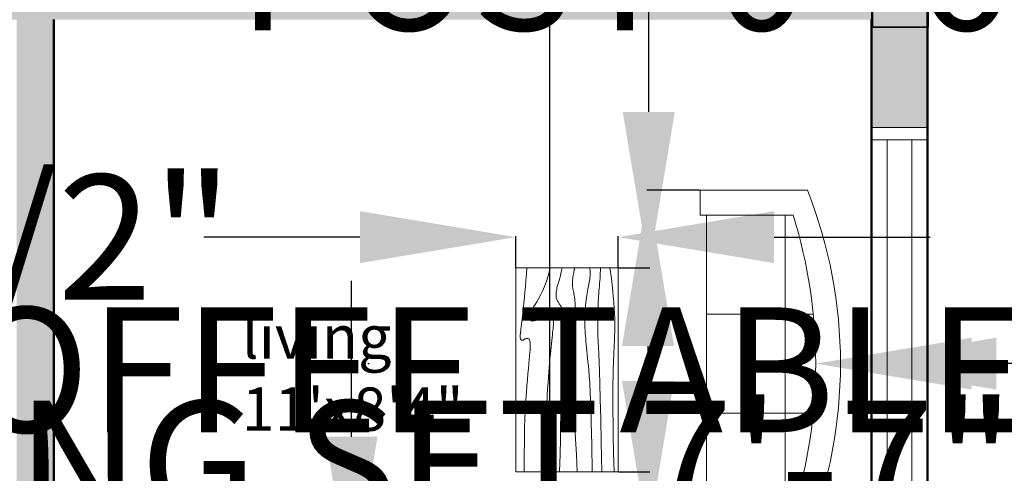
# Model space of a CAD drawing. Units: inches. Extents: x 25 to 82118, y 10 to 6494.
# Tile 6 of 9: x 40928 to 41087, y 3300 to 3373. Entities that reach past the tile are written whole.
import ezdxf

# ---------------------------------------------------------------- set-up
doc = ezdxf.new("R2010")
doc.units = ezdxf.units.IN
doc.header["$MEASUREMENT"] = 0
for name, color, linetype, lineweight in [('A-ANNO-DIMS', 2, 'Continuous', 18), ('A-AREA-IDEN', 7, 'Continuous', 25), ('A-FURN', 8, 'Continuous', 18), ('A-GLAZ', 4, 'Continuous', 18), ('A-WALL', 7, 'Continuous', 50)]:
    doc.layers.add(name, color=color, linetype=linetype, lineweight=lineweight)
doc.layers.add('A-COLS', color=30, linetype='Continuous', lineweight=35, true_color=0xf26722)
doc.layers.add('A-WALL-PATT', color=18, linetype='Continuous', lineweight=13, true_color=0x000000)
doc.styles.get("Standard").update_dxf_attribs({"font": 'arial.ttf'})
doc.dimstyles.get("Standard").update_dxf_attribs({"dimtxt": 20.18, "dimasz": 25.18, "dimexe": 0.18, "dimexo": 0.0625, "dimgap": 0.09, "dimtad": 0, "dimtih": 1, "dimtoh": 1, "dimdec": 0, "dimzin": 0, "dimdsep": 46, "dimlunit": 3, "dimtxsty": 'Standard', "dimcen": 0.09, "dimadec": 0, "dimazin": 0, "dimtfac": 1, "dimtdec": 0, "dimtofl": 0, "dimtmove": 0, "dimatfit": 3, "dimfxl": 1, "dimtolj": 1, "dimtzin": 0, "dimarcsym": 0})

# ---------------------------------------------------------------- blocks, each defined once
blk = doc.blocks.new('Table - Rectangular Woodgrain 60 x 30 in.')
for p, q in [((0, 0), (0, -30)), ((60, 0), (0, 0)), ((60, -30), (60, 0)), ((0, -30), (60, -30))]:
    blk.add_line(p, q)
for points in [[(0, -2.4), (4.8155, -2.418), (9.0302, -2.4688), (12.709, -2.5477), (15.9167, -2.65), (18.7181, -2.7711), (21.1781, -2.9063), (23.3616, -3.0508), (25.3333, -3.2), (27.1477, -3.3495), (28.8172, -3.4958), (30.3437, -3.636), (31.7291, -3.7667), (32.9756, -3.8849), (34.0849, -3.9875), (35.059, -4.0714), (35.9, -4.1334), (36.6114, -4.1711), (37.2041, -4.1854), (37.6906, -4.1779), (38.0833, -4.15), (38.3948, -4.1034), (38.6375, -4.0396), (38.8239, -3.9602), (38.9666, -3.8667), (39.0764, -3.7608), (39.1573, -3.6448), (39.2116, -3.521), (39.2416, -3.3917), (39.2498, -3.2593), (39.2385, -3.1261), (39.21, -2.9944), (39.1666, -2.8667), (39.111, -2.7447), (39.0468, -2.6281), (38.978, -2.5163), (38.9083, -2.4083), (38.8418, -2.3035), (38.7823, -2.201), (38.7337, -2.1001), (38.7, -2), (38.6844, -1.9003), (38.6875, -1.8021), (38.7094, -1.707), (38.75, -1.6167), (38.8094, -1.5326), (38.8875, -1.4563), (38.9844, -1.3893), (39.1, -1.3333), (39.2351, -1.2896), (39.3937, -1.2583), (39.5804, -1.2396), (39.8, -1.2333), (40.057, -1.2396), (40.3562, -1.2583), (40.7023, -1.2896), (41.1, -1.3333), (41.5547, -1.3895), (42.0755, -1.4573), (42.6721, -1.5361), (43.3542, -1.625), (44.1316, -1.7233), (45.014, -1.8302), (46.0114, -1.9449), (47.1333, -2.0667), (48.3862, -2.1947), (49.7625, -2.3281), (51.2513, -2.4663), (52.8416, -2.6083), (54.5226, -2.7535), (56.2833, -2.9011), (58.1127, -3.0501), (60, -3.2)], [(0, -9.2), (6.5759, -9.0858), (11.9385, -9.0365), (16.2527, -9.0418), (19.6833, -9.0917), (22.3952, -9.1759), (24.5531, -9.2844), (26.322, -9.4069), (27.8666, -9.5333), (29.3241, -9.6553), (30.7203, -9.7719), (32.0532, -9.8837), (33.3208, -9.9917), (34.5213, -10.0965), (35.6526, -10.199), (36.7128, -10.2999), (37.7, -10.4), (38.6129, -10.4996), (39.4531, -10.5969), (40.223, -10.6895), (40.925, -10.775), (41.5613, -10.8512), (42.1344, -10.9156), (42.6465, -10.966), (43.1, -11), (43.4976, -11.0158), (43.8437, -11.0136), (44.143, -10.9942), (44.4, -10.9583), (44.6195, -10.9069), (44.8062, -10.8406), (44.9648, -10.7603), (45.1, -10.6667), (45.2155, -10.5598), (45.3114, -10.4365), (45.3871, -10.2929), (45.4416, -10.125), (45.4743, -9.929), (45.4844, -9.7011), (45.4709, -9.4371), (45.4333, -9.1333), (45.3716, -8.7883), (45.2896, -8.4104), (45.1919, -8.0107), (45.0833, -7.6), (44.9685, -7.1893), (44.8521, -6.7896), (44.7388, -6.4117), (44.6333, -6.0667), (44.54, -5.7628), (44.4614, -5.4979), (44.4001, -5.2675), (44.3583, -5.0667), (44.3384, -4.8909), (44.3427, -4.7354), (44.3736, -4.5956), (44.4333, -4.4667), (44.5236, -4.3453), (44.6427, -4.2333), (44.7884, -4.1339), (44.9583, -4.05), (45.1501, -3.9849), (45.3614, -3.9417), (45.59, -3.9234), (45.8333, -3.9333), (46.0915, -3.9749), (46.3734, -4.0531), (46.6906, -4.1736), (47.0542, -4.3417), (47.4756, -4.5629), (47.9661, -4.8427), (48.5372, -5.1866), (49.2, -5.6), (49.9676, -6.0844), (50.8594, -6.625), (51.8965, -7.2031), (53.1, -7.8), (54.491, -8.3969), (56.0906, -8.975), (57.9199, -9.5156), (60, -10)], [(0, -12.8), (5.1847, -12.9322), (9.6213, -13.0323), (13.3963, -13.1059), (16.5958, -13.1583), (19.3063, -13.1952), (21.614, -13.2219), (23.6054, -13.2439), (25.3666, -13.2667), (26.9728, -13.2947), (28.4531, -13.3281), (29.8256, -13.3663), (31.1083, -13.4083), (32.3191, -13.4535), (33.476, -13.501), (34.597, -13.5501), (35.7, -13.6), (36.7984, -13.6497), (37.8875, -13.6979), (38.9578, -13.743), (40, -13.7833), (41.0047, -13.8174), (41.9625, -13.8438), (42.864, -13.8607), (43.7, -13.8667), (44.4631, -13.8604), (45.1552, -13.8417), (45.7801, -13.8104), (46.3416, -13.7667), (46.8439, -13.7104), (47.2906, -13.6417), (47.6858, -13.5604), (48.0333, -13.4667), (48.3375, -13.3608), (48.6042, -13.2448), (48.8396, -13.121), (49.05, -12.9917), (49.2417, -12.8593), (49.4208, -12.7261), (49.5937, -12.5944), (49.7667, -12.4667), (49.9452, -12.3451), (50.1323, -12.2313), (50.3303, -12.1268), (50.5416, -12.0333), (50.7686, -11.9524), (51.0135, -11.8854), (51.2788, -11.8341), (51.5666, -11.8), (51.8785, -11.7843), (52.2116, -11.7865), (52.562, -11.8059), (52.926, -11.8417), (53.2998, -11.8931), (53.6795, -11.9594), (54.0614, -12.0397), (54.4416, -12.1333), (54.8223, -12.2401), (55.2293, -12.3625), (55.6942, -12.5037), (56.2489, -12.6667), (56.9251, -12.8547), (57.7545, -13.0708), (58.7689, -13.3182), (60, -13.6)], [(0, -18), (5.124, -17.7273), (9.6609, -17.5057), (13.6705, -17.3303), (17.2125, -17.1958), (20.3467, -17.0973), (23.1328, -17.0297), (25.6307, -16.9878), (27.9, -16.9667), (29.9928, -16.9617), (31.9302, -16.9703), (33.7254, -16.9907), (35.3917, -17.0208), (36.9423, -17.0588), (38.3906, -17.1026), (39.7499, -17.1503), (41.0333, -17.2), (42.2519, -17.2496), (43.4073, -17.2969), (44.4986, -17.3395), (45.525, -17.375), (46.4858, -17.4012), (47.3802, -17.4156), (48.2074, -17.416), (48.9667, -17.4), (49.6583, -17.3662), (50.2872, -17.3167), (50.8595, -17.2547), (51.3812, -17.1833), (51.8584, -17.1057), (52.2971, -17.025), (52.7034, -16.9443), (53.0833, -16.8667), (53.443, -16.7951), (53.789, -16.7313), (54.128, -16.6768), (54.4666, -16.6334), (54.8115, -16.6024), (55.1693, -16.5854), (55.5465, -16.5841), (55.95, -16.6), (56.3828, -16.6337), (56.8346, -16.6823), (57.2915, -16.7418), (57.7396, -16.8084), (58.165, -16.878), (58.5539, -16.9469), (58.8924, -17.0111), (59.1666, -17.0667), (59.3679, -17.1107), (59.5078, -17.1438), (59.6032, -17.1675), (59.6708, -17.1833), (59.7275, -17.193), (59.7901, -17.1979), (59.8753, -17.1998), (60, -17.2)], [(0, -22.4), (8.0098, -22.2501), (14.4094, -22.1011), (19.4168, -21.9535), (23.25, -21.8083), (26.1269, -21.6663), (28.2656, -21.5281), (29.884, -21.3947), (31.2, -21.2667), (32.3967, -21.1448), (33.5172, -21.0292), (34.5697, -20.9198), (35.5625, -20.8167), (36.5037, -20.7198), (37.4015, -20.6292), (38.2642, -20.5448), (39.1, -20.4667), (39.9164, -20.3951), (40.7187, -20.3313), (41.5117, -20.2768), (42.3, -20.2333), (43.0883, -20.2024), (43.8812, -20.1854), (44.6836, -20.1841), (45.5, -20.2), (46.3328, -20.234), (47.1747, -20.2844), (48.0163, -20.3488), (48.8479, -20.425), (49.66, -20.5106), (50.4429, -20.6031), (51.1872, -20.7004), (51.8833, -20.8), (52.5246, -20.8999), (53.1166, -20.9995), (53.6681, -21.0983), (54.1875, -21.1958), (54.6834, -21.2919), (55.1646, -21.3859), (55.6394, -21.4777), (56.1167, -21.5667), (56.6028, -21.6515), (57.0961, -21.7266), (57.5929, -21.7852), (58.0896, -21.8208), (58.5823, -21.8268), (59.0674, -21.7964), (59.5412, -21.723), (60, -21.6)], [(0, -25.2), (8.6355, -25.0504), (15.7026, -24.9031), (21.4049, -24.7606), (25.9458, -24.625), (29.529, -24.4988), (32.3578, -24.3844), (34.6359, -24.284), (36.5667, -24.2), (38.3213, -24.1341), (39.9417, -24.0854), (41.437, -24.0523), (42.8167, -24.0333), (44.0901, -24.0268), (45.2667, -24.0313), (46.3557, -24.0451), (47.3667, -24.0667), (48.309, -24.0947), (49.1928, -24.1287), (50.0284, -24.168), (50.826, -24.2125), (51.5959, -24.2617), (52.3483, -24.3151), (53.0935, -24.3725), (53.8417, -24.4334), (54.6009, -24.497), (55.3699, -24.561), (56.1454, -24.6226), (56.9239, -24.6792), (57.7021, -24.7279), (58.4764, -24.7662), (59.2435, -24.7911), (60, -24.8)], [(0, -28.8), (5.6867, -28.6681), (10.45, -28.5698), (14.407, -28.5012), (17.675, -28.4584), (20.3711, -28.4374), (22.6125, -28.4344), (24.5164, -28.4455), (26.2, -28.4667), (27.762, -28.4947), (29.2276, -28.5281), (30.6033, -28.5663), (31.8958, -28.6084), (33.1118, -28.6535), (34.2578, -28.7011), (35.3405, -28.7501), (36.3666, -28.8), (37.3443, -28.8497), (38.288, -28.8974), (39.2137, -28.9412), (40.1375, -28.9792), (41.0753, -29.0093), (42.0432, -29.0297), (43.0572, -29.0384), (44.1333, -29.0333), (45.2936, -29.0114), (46.5843, -28.9641), (48.0579, -28.8816), (49.7666, -28.7542), (51.7629, -28.5721), (54.0989, -28.3255), (56.8272, -28.0048), (60, -27.6)]]:
    blk.add_lwpolyline(points)
blk = doc.blocks.new('Sofa - Roundback 7 ft.')
for p, q in [((-12.00002, -32.4421), (-12.00003, -6.5971)), ((11.99997, -32.4421), (11.99998, -6.5971)), ((-36.000027, -34), (-36.000027, -11.4696)), ((35.99998, -34), (35.99998, -11.4696)), ((-35.999844, -13.3819), (35.9998, -13.3819)), ((-36.000027, -32.4421), (35.99998, -32.4421))]:
    blk.add_line(p, q)
for points in [[(-36.000027, -34), (-42.000027, -34), (-42.000027, -8)], [(41.99998, -8), (41.99998, -34), (35.99998, -34)]]:
    blk.add_lwpolyline(points)
for centre, radius, start, end in [((0, -114.25), 114.25, 68.43141, 111.5686), ((-0.00001, -127.1968), 121.1968, 72.72033, 107.2797)]:
    blk.add_arc(centre, radius, start, end)
blk = doc.blocks.new('*D15')
at = {"layer": 'A-ANNO-DIMS', "color": 0, "lineweight": -2, "transparency": 16777216}
for p, q in [((41074.27, 3531.88), (41136.86, 3531.88)), ((41136.68, 3506.7), (41136.68, 3371.51)), ((41136.68, 3215.52), (41136.68, 3350.71)), ((41074.27, 3190.34), (41136.86, 3190.34))]:
    blk.add_line(p, q, dxfattribs=at)
at = {"layer": 'A-ANNO-DIMS', "color": 0, "transparency": 16777216}
for points in [[(41132.48, 3506.7), (41140.87, 3506.7), (41136.68, 3531.88)], [(41132.48, 3215.52), (41140.87, 3215.52), (41136.68, 3190.34)]]:
    blk.add_solid(points, dxfattribs=at)
at = {"layer": 'Defpoints', "color": 0, "transparency": 16777216}
for p in [(41074.21, 3531.88), (41074.21, 3190.34), (41136.68, 3190.34)]:
    blk.add_point(p, dxfattribs=at)
at = {"layer": 'A-ANNO-DIMS', "color": 0, "transparency": 16777216, "insert": (41136.68, 3361.11), "char_height": 20.18, "attachment_point": 5}
blk.add_mtext('\\A1;26\'3"', dxfattribs=at)
blk = doc.blocks.new('*D16')
at = {"layer": 'A-ANNO-DIMS', "color": 0, "lineweight": -2, "transparency": 16777216}
for p, q in [((41074.33, 3531.88), (41191.01, 3531.88)), ((41190.83, 3506.7), (41190.83, 3350.25)), ((41190.83, 3173), (41190.83, 3329.45)), ((41074.33, 3147.82), (41191.01, 3147.82))]:
    blk.add_line(p, q, dxfattribs=at)
at = {"layer": 'A-ANNO-DIMS', "color": 0, "transparency": 16777216}
for points in [[(41186.63, 3506.7), (41195.02, 3506.7), (41190.83, 3531.88)], [(41186.63, 3173), (41195.02, 3173), (41190.83, 3147.82)]]:
    blk.add_solid(points, dxfattribs=at)
at = {"layer": 'Defpoints', "color": 0, "transparency": 16777216}
for p in [(41074.27, 3531.88), (41074.27, 3147.82), (41190.83, 3147.82)]:
    blk.add_point(p, dxfattribs=at)
at = {"layer": 'A-ANNO-DIMS', "color": 0, "transparency": 16777216, "insert": (41190.83, 3339.85), "char_height": 20.18, "attachment_point": 5}
blk.add_mtext("\\A1;32'", dxfattribs=at)
blk = doc.blocks.new('WIN-72IN-9W')
for p, q in [((9, 76), (0, 76)), ((9, 74), (0, 74)), ((2.5, 74), (2.5, 2)), ((6.5, 74), (6.5, 2)), ((9, 2), (0, 2)), ((9, 0), (0, 0))]:
    blk.add_line(p, q)
blk = doc.blocks.new('COL-9X9')
h = blk.add_hatch(color=256)
h.dxf.hatch_style = 1
h.paths.add_polyline_path([(9, 9), (0, 9), (0, 0), (9, 0)])
blk.add_lwpolyline([(0, 0), (9, 0), (9, 9), (0, 9)], close=True)
blk = doc.blocks.new('*D25')
at = {"layer": 'A-ANNO-DIMS', "color": 0, "lineweight": -2, "transparency": 16777216}
for p, q in [((40724.56, 3429.21), (40724.56, 3454.39)), ((40724.56, 3454.39), (40749.74, 3454.39)), ((40723.27, 3404.03), (40724.74, 3404.03)), ((40723.27, 3395.03), (40724.74, 3395.03)), ((40724.56, 3369.85), (40724.56, 3344.67))]:
    blk.add_line(p, q, dxfattribs=at)
at = {"layer": 'A-ANNO-DIMS', "color": 0, "transparency": 16777216}
for points in [[(40720.36, 3429.21), (40728.76, 3429.21), (40724.56, 3404.03)], [(40720.36, 3369.85), (40728.76, 3369.85), (40724.56, 3395.03)]]:
    blk.add_solid(points, dxfattribs=at)
at = {"layer": 'Defpoints', "color": 0, "transparency": 16777216}
for p in [(40723.21, 3404.03), (40724.56, 3404.03), (40723.21, 3395.03)]:
    blk.add_point(p, dxfattribs=at)
at = {"layer": 'A-ANNO-DIMS', "color": 0, "transparency": 16777216, "insert": (40876.22, 3454.39), "char_height": 20.18, "attachment_point": 5}
blk.add_mtext('\\A1;COLUMN 0\'-9" TYP.', dxfattribs=at)
blk = doc.blocks.new('*D27')
at = {"layer": 'A-ANNO-DIMS', "color": 0, "lineweight": -2, "transparency": 16777216}
for p, q in [((40903.21, 3382.03), (40903.21, 3381.02)), ((40909.21, 3382.03), (40909.21, 3381.02)), ((40878.03, 3381.2), (40852.85, 3381.2)), ((40934.39, 3381.2), (40959.57, 3381.2))]:
    blk.add_line(p, q, dxfattribs=at)
at = {"layer": 'A-ANNO-DIMS', "color": 0, "transparency": 16777216}
for points in [[(40878.03, 3385.39), (40878.03, 3377), (40903.21, 3381.2)], [(40934.39, 3385.39), (40934.39, 3377), (40909.21, 3381.2)]]:
    blk.add_solid(points, dxfattribs=at)
at = {"layer": 'Defpoints', "color": 0, "transparency": 16777216}
for p in [(40903.21, 3382.1), (40909.21, 3382.1), (40909.21, 3381.2)]:
    blk.add_point(p, dxfattribs=at)
at = {"layer": 'A-ANNO-DIMS', "color": 0, "transparency": 16777216, "insert": (41062.95, 3381.2), "char_height": 20.18, "attachment_point": 5}
blk.add_mtext('\\A1;POST 0\'-6" TYP.', dxfattribs=at)
blk = doc.blocks.new('*D28')
at = {"layer": 'A-ANNO-DIMS', "color": 0, "lineweight": -2, "transparency": 16777216}
for p, q in [((40910.11, 3413.07), (40910.11, 3438.25)), ((40910.11, 3438.25), (40935.29, 3438.25)), ((40909.27, 3387.89), (40910.29, 3387.89)), ((40909.27, 3382.1), (40910.29, 3382.1)), ((40910.11, 3356.92), (40910.11, 3331.74))]:
    blk.add_line(p, q, dxfattribs=at)
at = {"layer": 'A-ANNO-DIMS', "color": 0, "transparency": 16777216}
for points in [[(40905.91, 3413.07), (40914.31, 3413.07), (40910.11, 3387.89)], [(40905.91, 3356.92), (40914.31, 3356.92), (40910.11, 3382.1)]]:
    blk.add_solid(points, dxfattribs=at)
at = {"layer": 'Defpoints', "color": 0, "transparency": 16777216}
for p in [(40909.21, 3387.89), (40910.11, 3387.89), (40909.21, 3382.1)]:
    blk.add_point(p, dxfattribs=at)
at = {"layer": 'A-ANNO-DIMS', "color": 0, "transparency": 16777216, "insert": (40996.88, 3438.25), "char_height": 20.18, "attachment_point": 5}
blk.add_mtext('\\A1;0\'-6" TYP.', dxfattribs=at)
blk = doc.blocks.new('*D43')
at = {"layer": 'A-ANNO-DIMS', "color": 0, "lineweight": -2, "transparency": 16777216}
for p, q in [((41029.25, 3357.91), (41029.25, 3383.09)), ((41024.37, 3332.73), (41029.43, 3332.73)), ((41024.37, 3299.75), (41029.43, 3299.75)), ((41029.25, 3274.57), (41029.25, 3249.39))]:
    blk.add_line(p, q, dxfattribs=at)
at = {"layer": 'A-ANNO-DIMS', "color": 0, "transparency": 16777216}
for points in [[(41025.05, 3357.91), (41033.45, 3357.91), (41029.25, 3332.73)], [(41025.05, 3274.57), (41033.45, 3274.57), (41029.25, 3299.75)]]:
    blk.add_solid(points, dxfattribs=at)
at = {"layer": 'Defpoints', "color": 0, "transparency": 16777216}
for p in [(41024.3, 3332.73), (41029.25, 3332.73), (41024.3, 3299.75)]:
    blk.add_point(p, dxfattribs=at)
at = {"layer": 'A-ANNO-DIMS', "color": 0, "transparency": 16777216, "insert": (41029.25, 3316.24), "char_height": 20.18, "attachment_point": 5}
blk.add_mtext('\\A1;COFFEE TABLE 2\'-9"', dxfattribs=at)
blk = doc.blocks.new('*D44')
at = {"layer": 'A-ANNO-DIMS', "color": 0, "lineweight": -2, "transparency": 16777216}
for p, q in [((40982.63, 3337.68), (40957.45, 3337.68)), ((41007.81, 3332.8), (41007.81, 3337.86)), ((41024.3, 3332.8), (41024.3, 3337.86)), ((41049.48, 3337.68), (41074.66, 3337.68))]:
    blk.add_line(p, q, dxfattribs=at)
at = {"layer": 'A-ANNO-DIMS', "color": 0, "transparency": 16777216}
for points in [[(40982.63, 3341.88), (40982.63, 3333.48), (41007.81, 3337.68)], [(41049.48, 3341.88), (41049.48, 3333.48), (41024.3, 3337.68)]]:
    blk.add_solid(points, dxfattribs=at)
at = {"layer": 'Defpoints', "color": 0, "transparency": 16777216}
for p in [(41007.81, 3337.68), (41007.81, 3332.73), (41024.3, 3332.73)]:
    blk.add_point(p, dxfattribs=at)
at = {"layer": 'A-ANNO-DIMS', "color": 0, "transparency": 16777216, "insert": (40907.98, 3337.68), "char_height": 20.18, "attachment_point": 5}
blk.add_mtext('\\A1;1\'-4 1/2"', dxfattribs=at)
blk = doc.blocks.new('*D45')
at = {"layer": 'A-ANNO-DIMS', "color": 0, "lineweight": -2, "transparency": 16777216}
for p, q in [((41037.46, 3345.25), (41028.94, 3345.25)), ((41029.12, 3320.07), (41029.12, 3314.42)), ((41037.46, 3289.24), (41028.94, 3289.24)), ((41029.12, 3289.24), (41029.12, 3264.06)), ((41029.12, 3264.06), (41003.94, 3264.06))]:
    blk.add_line(p, q, dxfattribs=at)
at = {"layer": 'A-ANNO-DIMS', "color": 0, "transparency": 16777216}
for points in [[(41024.92, 3320.07), (41033.32, 3320.07), (41029.12, 3345.25)], [(41024.92, 3314.42), (41033.32, 3314.42), (41029.12, 3289.24)]]:
    blk.add_solid(points, dxfattribs=at)
at = {"layer": 'Defpoints', "color": 0, "transparency": 16777216}
for p in [(41037.52, 3345.25), (41029.12, 3289.24), (41037.52, 3289.24)]:
    blk.add_point(p, dxfattribs=at)
at = {"layer": 'A-ANNO-DIMS', "color": 0, "transparency": 16777216, "insert": (40934.78, 3264.06), "char_height": 20.18, "attachment_point": 5}
blk.add_mtext('\\A1;SOFA 4\'-8"', dxfattribs=at)
blk = doc.blocks.new('*D46')
at = {"layer": 'A-ANNO-DIMS', "color": 0, "lineweight": -2, "transparency": 16777216}
for p, q in [((41037.52, 3289.18), (41037.52, 3280.66)), ((41061.97, 3289.18), (41061.97, 3280.66)), ((41012.34, 3280.84), (40987.16, 3280.84)), ((41087.15, 3280.84), (41112.33, 3280.84))]:
    blk.add_line(p, q, dxfattribs=at)
at = {"layer": 'A-ANNO-DIMS', "color": 0, "transparency": 16777216}
for points in [[(41012.34, 3285.04), (41012.34, 3276.64), (41037.52, 3280.84)], [(41087.15, 3285.04), (41087.15, 3276.64), (41061.97, 3280.84)]]:
    blk.add_solid(points, dxfattribs=at)
at = {"layer": 'Defpoints', "color": 0, "transparency": 16777216}
for p in [(41037.52, 3289.24), (41061.97, 3289.24), (41061.97, 3280.84)]:
    blk.add_point(p, dxfattribs=at)
at = {"layer": 'A-ANNO-DIMS', "color": 0, "transparency": 16777216, "insert": (41162.92, 3280.84), "char_height": 20.18, "attachment_point": 5}
blk.add_mtext('\\A1;2\'-0 1/2"', dxfattribs=at)
blk = doc.blocks.new('*D47')
at = {"layer": 'A-ANNO-DIMS', "color": 0, "lineweight": -2, "transparency": 16777216}
for p, q in [((40753.09, 3314.74), (40753.09, 3300.97)), ((40844.09, 3314.74), (40844.09, 3300.97)), ((40778.27, 3301.15), (40818.91, 3301.15)), ((40844.09, 3301.15), (40869.27, 3301.15))]:
    blk.add_line(p, q, dxfattribs=at)
at = {"layer": 'A-ANNO-DIMS', "color": 0, "transparency": 16777216}
for points in [[(40778.27, 3305.35), (40778.27, 3296.95), (40753.09, 3301.15)], [(40818.91, 3305.35), (40818.91, 3296.95), (40844.09, 3301.15)]]:
    blk.add_solid(points, dxfattribs=at)
at = {"layer": 'Defpoints', "color": 0, "transparency": 16777216}
for p in [(40753.09, 3314.8), (40844.09, 3314.8), (40844.09, 3301.15)]:
    blk.add_point(p, dxfattribs=at)
at = {"layer": 'A-ANNO-DIMS', "color": 0, "transparency": 16777216, "insert": (40980.26, 3301.15), "char_height": 20.18, "attachment_point": 5}
blk.add_mtext('\\A1;DINING SET 7\'-7"', dxfattribs=at)
blk = doc.blocks.new('*D48')
at = {"layer": 'A-ANNO-DIMS', "color": 0, "lineweight": -2, "transparency": 16777216}
for p, q in [((40857.74, 3369.8), (40857.74, 3394.98)), ((40857.74, 3394.98), (40882.92, 3394.98)), ((40844.15, 3369.8), (40857.92, 3369.8)), ((40857.74, 3339.98), (40857.74, 3344.62)), ((40844.15, 3314.8), (40857.92, 3314.8))]:
    blk.add_line(p, q, dxfattribs=at)
at = {"layer": 'A-ANNO-DIMS', "color": 0, "transparency": 16777216}
for points in [[(40853.54, 3344.62), (40861.93, 3344.62), (40857.74, 3369.8)], [(40853.54, 3339.98), (40861.93, 3339.98), (40857.74, 3314.8)]]:
    blk.add_solid(points, dxfattribs=at)
at = {"layer": 'Defpoints', "color": 0, "transparency": 16777216}
for p in [(40844.09, 3369.8), (40857.74, 3369.8), (40844.09, 3314.8)]:
    blk.add_point(p, dxfattribs=at)
at = {"layer": 'A-ANNO-DIMS', "color": 0, "transparency": 16777216, "insert": (40910.23, 3394.98), "char_height": 20.18, "attachment_point": 5}
blk.add_mtext('\\A1;4\'-7"', dxfattribs=at)
blk = doc.blocks.new('*D49')
at = {"layer": 'A-ANNO-DIMS', "color": 0, "lineweight": -2, "transparency": 16777216}
for p, q in [((40987.49, 3280.33), (40987.49, 3286.67)), ((41028.96, 3280.33), (41028.96, 3286.67)), ((40962.31, 3286.49), (40937.13, 3286.49)), ((41054.14, 3286.49), (41079.32, 3286.49))]:
    blk.add_line(p, q, dxfattribs=at)
at = {"layer": 'A-ANNO-DIMS', "color": 0, "transparency": 16777216}
for points in [[(40962.31, 3290.68), (40962.31, 3282.29), (40987.49, 3286.49)], [(41054.14, 3290.68), (41054.14, 3282.29), (41028.96, 3286.49)]]:
    blk.add_solid(points, dxfattribs=at)
at = {"layer": 'Defpoints', "color": 0, "transparency": 16777216}
for p in [(40987.49, 3286.49), (40987.49, 3280.26), (41028.96, 3280.26)]:
    blk.add_point(p, dxfattribs=at)
at = {"layer": 'A-ANNO-DIMS', "color": 0, "transparency": 16777216, "insert": (40808.81, 3286.49), "char_height": 20.18, "attachment_point": 5}
blk.add_mtext('\\A1;LOVESEAT 3\'-5 1/2"', dxfattribs=at)
blk = doc.blocks.new('*D50')
at = {"layer": 'A-ANNO-DIMS', "color": 0, "lineweight": -2, "transparency": 16777216}
for p, q in [((40981.27, 3305.44), (40981.27, 3330.62)), ((40987.43, 3280.26), (40981.09, 3280.26)), ((40987.43, 3254.92), (40981.09, 3254.92)), ((40981.27, 3229.74), (40981.27, 3204.56))]:
    blk.add_line(p, q, dxfattribs=at)
at = {"layer": 'A-ANNO-DIMS', "color": 0, "transparency": 16777216}
for points in [[(40977.07, 3305.44), (40985.46, 3305.44), (40981.27, 3280.26)], [(40977.07, 3229.74), (40985.46, 3229.74), (40981.27, 3254.92)]]:
    blk.add_solid(points, dxfattribs=at)
at = {"layer": 'Defpoints', "color": 0, "transparency": 16777216}
for p in [(40987.49, 3280.26), (40981.27, 3254.92), (40987.49, 3254.92)]:
    blk.add_point(p, dxfattribs=at)
at = {"layer": 'A-ANNO-DIMS', "color": 0, "transparency": 16777216, "insert": (40981.27, 3267.59), "char_height": 20.18, "attachment_point": 5}
blk.add_mtext('\\A1;2\'-1 1/2"', dxfattribs=at)
blk = doc.blocks.new('*D65')
at = {"layer": 'A-ANNO-DIMS', "color": 0, "lineweight": -2, "transparency": 16777216}
for p, q in [((41102.56, 3304.59), (41102.56, 3329.77)), ((41065.27, 3279.41), (41102.74, 3279.41)), ((41065.27, 3246.82), (41102.74, 3246.82)), ((41102.56, 3221.64), (41102.56, 3196.46))]:
    blk.add_line(p, q, dxfattribs=at)
at = {"layer": 'A-ANNO-DIMS', "color": 0, "transparency": 16777216}
for points in [[(41098.36, 3304.59), (41106.76, 3304.59), (41102.56, 3279.41)], [(41098.36, 3221.64), (41106.76, 3221.64), (41102.56, 3246.82)]]:
    blk.add_solid(points, dxfattribs=at)
at = {"layer": 'Defpoints', "color": 0, "transparency": 16777216}
for p in [(41065.21, 3279.41), (41102.56, 3279.41), (41065.21, 3246.82)]:
    blk.add_point(p, dxfattribs=at)
at = {"layer": 'A-ANNO-DIMS', "color": 0, "transparency": 16777216, "insert": (41102.56, 3263.11), "char_height": 20.18, "attachment_point": 5}
blk.add_mtext('\\A1;2\'-8 1/2"', dxfattribs=at)
blk = doc.blocks.new('*D66')
at = {"layer": 'A-ANNO-DIMS', "color": 0, "lineweight": -2, "transparency": 16777216}
for p, q in [((41013.21, 3522.76), (41013.21, 3119.41)), ((41065.21, 3522.76), (41065.21, 3119.41)), ((41038.39, 3119.59), (41040.03, 3119.59)), ((41065.21, 3119.59), (41090.39, 3119.59))]:
    blk.add_line(p, q, dxfattribs=at)
at = {"layer": 'A-ANNO-DIMS', "color": 0, "transparency": 16777216}
for points in [[(41038.39, 3123.78), (41038.39, 3115.39), (41013.21, 3119.59)], [(41040.03, 3123.78), (41040.03, 3115.39), (41065.21, 3119.59)]]:
    blk.add_solid(points, dxfattribs=at)
at = {"layer": 'Defpoints', "color": 0, "transparency": 16777216}
for p in [(41013.21, 3522.82), (41065.21, 3522.82), (41065.21, 3119.59)]:
    blk.add_point(p, dxfattribs=at)
at = {"layer": 'A-ANNO-DIMS', "color": 0, "transparency": 16777216, "insert": (41117.71, 3119.59), "char_height": 20.18, "attachment_point": 5}
blk.add_mtext('\\A1;4\'-4"', dxfattribs=at)
blk = doc.blocks.new('*D67')
at = {"layer": 'A-ANNO-DIMS', "color": 0, "lineweight": -2, "transparency": 16777216}
for p, q in [((40770.03, 3572.85), (40744.85, 3572.85)), ((40795.21, 3156.88), (40795.21, 3573.03)), ((40838.63, 3156.88), (40838.63, 3573.03)), ((40863.81, 3572.85), (40888.99, 3572.85))]:
    blk.add_line(p, q, dxfattribs=at)
at = {"layer": 'A-ANNO-DIMS', "color": 0, "transparency": 16777216}
for points in [[(40770.03, 3577.05), (40770.03, 3568.66), (40795.21, 3572.85)], [(40863.81, 3577.05), (40863.81, 3568.66), (40838.63, 3572.85)]]:
    blk.add_solid(points, dxfattribs=at)
at = {"layer": 'Defpoints', "color": 0, "transparency": 16777216}
for p in [(40838.63, 3572.85), (40795.21, 3156.82), (40838.63, 3156.82)]:
    blk.add_point(p, dxfattribs=at)
at = {"layer": 'A-ANNO-DIMS', "color": 0, "transparency": 16777216, "insert": (40939.41, 3572.85), "char_height": 20.18, "attachment_point": 5}
blk.add_mtext('\\A1;3\'-7 1/2"', dxfattribs=at)
blk = doc.blocks.new('*D69')
at = {"layer": 'A-ANNO-DIMS', "color": 0, "lineweight": -2, "transparency": 16777216}
for p, q in [((40975.29, 3317.24), (40975.47, 3317.24)), ((40975.38, 3317.15), (40975.38, 3317.33)), ((41106.55, 3317.24), (41081.37, 3317.24))]:
    blk.add_line(p, q, dxfattribs=at)
at = {"layer": 'A-ANNO-DIMS', "color": 0, "transparency": 16777216}
blk.add_solid([(41081.37, 3321.44), (41081.37, 3313.05), (41056.19, 3317.24)], dxfattribs=at)
at = {"layer": 'Defpoints', "color": 0, "transparency": 16777216}
for p in [(40975.38, 3317.24), (41056.19, 3317.24)]:
    blk.add_point(p, dxfattribs=at)
at = {"layer": 'A-ANNO-DIMS', "color": 0, "transparency": 16777216, "insert": (41143.12, 3317.24), "char_height": 20.18, "attachment_point": 5}
blk.add_mtext('\\A1;R6\'-9"', dxfattribs=at)
blk = doc.blocks.new('*D70')
at = {"layer": 'A-ANNO-DIMS', "color": 0, "lineweight": -2, "transparency": 16777216}
for p, q in [((40983.92, 3317.24), (40984.1, 3317.24)), ((40984.01, 3317.15), (40984.01, 3317.33)), ((41110.55, 3317.24), (41085.37, 3317.24))]:
    blk.add_line(p, q, dxfattribs=at)
at = {"layer": 'A-ANNO-DIMS', "color": 0, "transparency": 16777216}
blk.add_solid([(41085.37, 3321.44), (41085.37, 3313.05), (41060.19, 3317.24)], dxfattribs=at)
at = {"layer": 'Defpoints', "color": 0, "transparency": 16777216}
for p in [(40984.01, 3317.24), (41060.19, 3317.24)]:
    blk.add_point(p, dxfattribs=at)
at = {"layer": 'A-ANNO-DIMS', "color": 0, "transparency": 16777216, "insert": (41147.12, 3317.24), "char_height": 20.18, "attachment_point": 5}
blk.add_mtext('\\A1;R6\'-4"', dxfattribs=at)

msp = doc.modelspace()

# ---------------------------------------------------------------- hatches: boundary and pattern name
at = {"layer": 'A-WALL-PATT'}
h = msp.add_hatch(color=256, dxfattribs=at)
h.dxf.hatch_style = 1
h.paths.add_polyline_path([(40778.43, 3531.82), (40723.21, 3531.82), (40723.21, 3522.82), (40778.54, 3522.82, -0.01877), (40778.43, 3525.82)])
h.paths.add_polyline_path([(40723.21, 3522.82), (40714.21, 3522.82), (40714.21, 3500.82), (40723.21, 3500.82)])
h.paths.add_polyline_path([(40723.21, 3424.82), (40714.21, 3424.82), (40714.21, 3404.03), (40723.21, 3404.03)])
h.paths.add_polyline_path([(40723.21, 3395.03), (40714.21, 3395.03), (40714.21, 3386.82), (40723.21, 3386.82)])
h.paths.add_polyline_path([(40901.65, 3531.82), (40834.16, 3531.82), (40834.16, 3522.82), (40901.65, 3522.82)])
h.paths.add_polyline_path([(40825.16, 3531.82), (40818.43, 3531.82), (40818.43, 3525.82), (40818.43, 3522.82), (40825.16, 3522.82)])
h.paths.add_polyline_path([(40961.21, 3531.82), (40910.65, 3531.82), (40910.65, 3522.82), (40961.21, 3522.82)])
h.paths.add_polyline_path([(41065.21, 3531.82), (41013.21, 3531.82), (41013.21, 3522.82), (41065.21, 3522.82)])
h.paths.add_polyline_path([(41074.21, 3522.82), (41065.21, 3522.82), (41065.21, 3506.52), (41074.21, 3506.52)])
h.paths.add_polyline_path([(41074.21, 3430.52), (41065.21, 3430.52), (41065.21, 3428.74), (41065.21, 3380.62), (41074.21, 3380.62)])
h.paths.add_polyline_path([(41074.21, 3371.62), (41065.21, 3371.62), (41065.21, 3355.41), (41074.21, 3355.41)])
h.paths.add_polyline_path([(41065.36, 3378.82), (40909.21, 3378.82), (40909.21, 3382.1), (40903.21, 3382.1), (40903.21, 3372.82), (41065.36, 3372.82)])
h.paths.add_polyline_path([(40933.21, 3372.82), (40927.21, 3372.82), (40927.21, 3282.62), (40933.21, 3282.62)])
h.paths.add_polyline_path([(41074.21, 3279.41), (41065.21, 3279.41), (41065.21, 3240.82), (41074.21, 3240.82)])
h.paths.add_polyline_path([(41065.21, 3246.82), (41052.05, 3246.82), (41052.05, 3240.82), (41065.21, 3240.82)])
h.paths.add_polyline_path([(40985.75, 3202.89), (41023.1, 3202.89), (41023.1, 3229.01), (40985.75, 3229.01)], flags=9)
h.paths.add_polyline_path([(40960.75, 3302.54), (40998.1, 3302.54), (40998.1, 3328.66), (40960.75, 3328.66)], flags=9)

# ---------------------------------------------------------------- linework, layer by layer
at = {"layer": 'A-WALL'}
for p, q in [((41074.21, 3531.82), (41074.21, 3147.82)), ((40933.21, 3372.82), (40933.21, 3246.82)), ((41065.21, 3372.82), (41065.21, 3240.82))]:
    msp.add_line(p, q, dxfattribs=at)

# ---------------------------------------------------------------- block references
at = {"layer": 'A-COLS', "rotation": 89.99999999995948}
msp.add_blockref('COL-9X9', (41074.36, 3371.62), dxfattribs=at)
at = {"layer": 'A-FURN'}
for name, p, xscale, yscale, zscale, rotation in [('Sofa - Roundback 7 ft.', (41060.19, 3317.24), 0.666763508743389, 0.666763508743389, 0.666763508743389, 270), ('Table - Rectangular Woodgrain 60 x 30 in.', (41007.81, 3299.75), 0.5497099540793171, 0.5497099540793171, 0.5497099540793171, 90)]:
    msp.add_blockref(name, p, dxfattribs=dict(at, xscale=xscale, yscale=yscale, zscale=zscale, rotation=rotation))
at = {"layer": 'A-GLAZ'}
msp.add_blockref('WIN-72IN-9W', (41065.21, 3279.41), dxfattribs=at)

# ---------------------------------------------------------------- texts
at = {"layer": 'A-AREA-IDEN', "insert": (40963.56, 3325.06), "char_height": 7, "attachment_point": 1}
msp.add_mtext_dynamic_manual_height_columns('living\\P11\'x8\'4"', width=132.9687, gutter_width=1, heights=[0], dxfattribs=at)

# ---------------------------------------------------------------- dimensions: what is measured, and where the dimension line sits
at = {"layer": 'A-ANNO-DIMS'}
for base, p1, p2, picture, middle in [((40838.63, 3572.85), (40795.21, 3156.82), (40838.63, 3156.82), '*D67', (40939.41, 3572.85)), ((41065.21, 3119.59), (41013.21, 3522.82), (41065.21, 3522.82), '*D66', (41117.71, 3119.59)), ((41061.9692, 3280.8387), (41037.5212, 3289.2399), (41061.9692, 3289.2399), '*D46', (41162.9243, 3280.8387))]:
    dim = msp.add_linear_dim(base=base, p1=p1, p2=p2, dimstyle='Standard', override={"dimdec": 1, "dimlfac": 1, "dimrnd": 0, "dimzin": 1, "dimdsep": 46, "dimlunit": 4, "dimfrac": 2}, dxfattribs=at)
    dim.commit()
    dim.dimension.update_dxf_attribs({"geometry": picture, "text_midpoint": middle})
for base, p1, p2, angle, text, override, picture, middle in [((41136.68, 3190.34), (41074.21, 3531.88), (41074.21, 3190.34), 90, '26\'3"', {"dimclrd": 0, "dimclre": 0, "dimclrt": 0}, '*D15', (41136.68, 3361.11)), ((40724.56, 3404.03), (40723.21, 3395.03), (40723.21, 3404.03), 90, 'COLUMN <> TYP.', {"dimdec": 1, "dimlfac": 1, "dimrnd": 0, "dimzin": 1, "dimdsep": 46, "dimlunit": 4, "dimfrac": 2}, '*D25', (40876.22, 3454.39)), ((40910.11, 3387.89), (40909.21, 3382.1), (40909.21, 3387.89), 90, '<> TYP.', {"dimdec": 1, "dimlfac": 1, "dimrnd": 0, "dimzin": 1, "dimdsep": 46, "dimlunit": 4, "dimfrac": 2}, '*D28', (40996.88, 3438.25)), ((41029.25, 3332.73), (41024.3, 3299.75), (41024.3, 3332.73), 90, 'COFFEE TABLE <>', {"dimdec": 1, "dimlfac": 1, "dimrnd": 0, "dimzin": 1, "dimdsep": 46, "dimlunit": 4, "dimfrac": 2}, '*D43', (41029.25, 3316.24)), ((41029.12, 3289.24), (41037.52, 3345.25), (41037.52, 3289.24), 270, 'SOFA <>', {"dimdec": 1, "dimlfac": 1, "dimrnd": 0, "dimzin": 1, "dimdsep": 46, "dimlunit": 4, "dimfrac": 2}, '*D45', (40934.78, 3264.06)), ((40987.49, 3286.49), (41028.96, 3280.26), (40987.49, 3280.26), 180, 'LOVESEAT <>', {"dimdec": 1, "dimlfac": 1, "dimrnd": 0, "dimzin": 1, "dimdsep": 46, "dimlunit": 4, "dimfrac": 2}, '*D49', (40808.81, 3286.49))]:
    dim = msp.add_linear_dim(base=base, p1=p1, p2=p2, angle=angle, text=text, dimstyle='Standard', override=override, dxfattribs=at)
    dim.commit()
    dim.dimension.update_dxf_attribs({"geometry": picture, "text_midpoint": middle})
for base, p1, p2, angle, override, picture, middle in [((41190.83, 3147.82), (41074.27, 3531.88), (41074.27, 3147.82), 90, {"dimclrd": 0, "dimclre": 0, "dimclrt": 0}, '*D16', (41190.83, 3339.85)), ((40857.74, 3369.8), (40844.09, 3314.8), (40844.09, 3369.8), 90, {"dimdec": 1, "dimlfac": 1, "dimrnd": 0, "dimzin": 1, "dimdsep": 46, "dimlunit": 4, "dimfrac": 2}, '*D48', (40910.23, 3394.98)), ((41007.81, 3337.68), (41024.3, 3332.73), (41007.81, 3332.73), 180, {"dimdec": 1, "dimlfac": 1, "dimrnd": 0, "dimzin": 1, "dimdsep": 46, "dimlunit": 4, "dimfrac": 2}, '*D44', (40907.98, 3337.68)), ((40981.27, 3254.92), (40987.49, 3280.26), (40987.49, 3254.92), 270, {"dimdec": 1, "dimlfac": 1, "dimrnd": 0, "dimzin": 1, "dimdsep": 46, "dimlunit": 4, "dimfrac": 2}, '*D50', (40981.27, 3267.59)), ((41102.56, 3279.41), (41065.21, 3246.82), (41065.21, 3279.41), 90, {"dimdec": 1, "dimlfac": 1, "dimrnd": 0, "dimzin": 1, "dimdsep": 46, "dimlunit": 4, "dimfrac": 2}, '*D65', (41102.56, 3263.11))]:
    dim = msp.add_linear_dim(base=base, p1=p1, p2=p2, angle=angle, dimstyle='Standard', override=override, dxfattribs=at)
    dim.commit()
    dim.dimension.update_dxf_attribs({"geometry": picture, "text_midpoint": middle})
for base, p1, p2, text, picture, middle in [((40909.21, 3381.2), (40903.21, 3382.1), (40909.21, 3382.1), 'POST <> TYP.', '*D27', (41062.95, 3381.2)), ((40844.09, 3301.15), (40753.09, 3314.8), (40844.09, 3314.8), 'DINING SET <>', '*D47', (40980.26, 3301.15))]:
    dim = msp.add_linear_dim(base=base, p1=p1, p2=p2, text=text, dimstyle='Standard', override={"dimdec": 1, "dimlfac": 1, "dimrnd": 0, "dimzin": 1, "dimdsep": 46, "dimlunit": 4, "dimfrac": 2}, dxfattribs=at)
    dim.commit()
    dim.dimension.update_dxf_attribs({"geometry": picture, "text_midpoint": middle})
for center, mpoint, picture, middle in [((40975.38, 3317.24), (41056.19, 3317.24), '*D69', (41143.12, 3317.24)), ((40984.01, 3317.24), (41060.19, 3317.24), '*D70', (41147.12, 3317.24))]:
    dim = msp.add_radius_dim(center=center, mpoint=mpoint, dimstyle='Standard', override={"dimdec": 1, "dimlfac": 1, "dimrnd": 0, "dimzin": 1, "dimdsep": 46, "dimlunit": 4, "dimfrac": 2}, dxfattribs=at)
    dim.commit()
    dim.dimension.update_dxf_attribs({"geometry": picture, "text_midpoint": middle})

doc.saveas('drawing.dxf')
